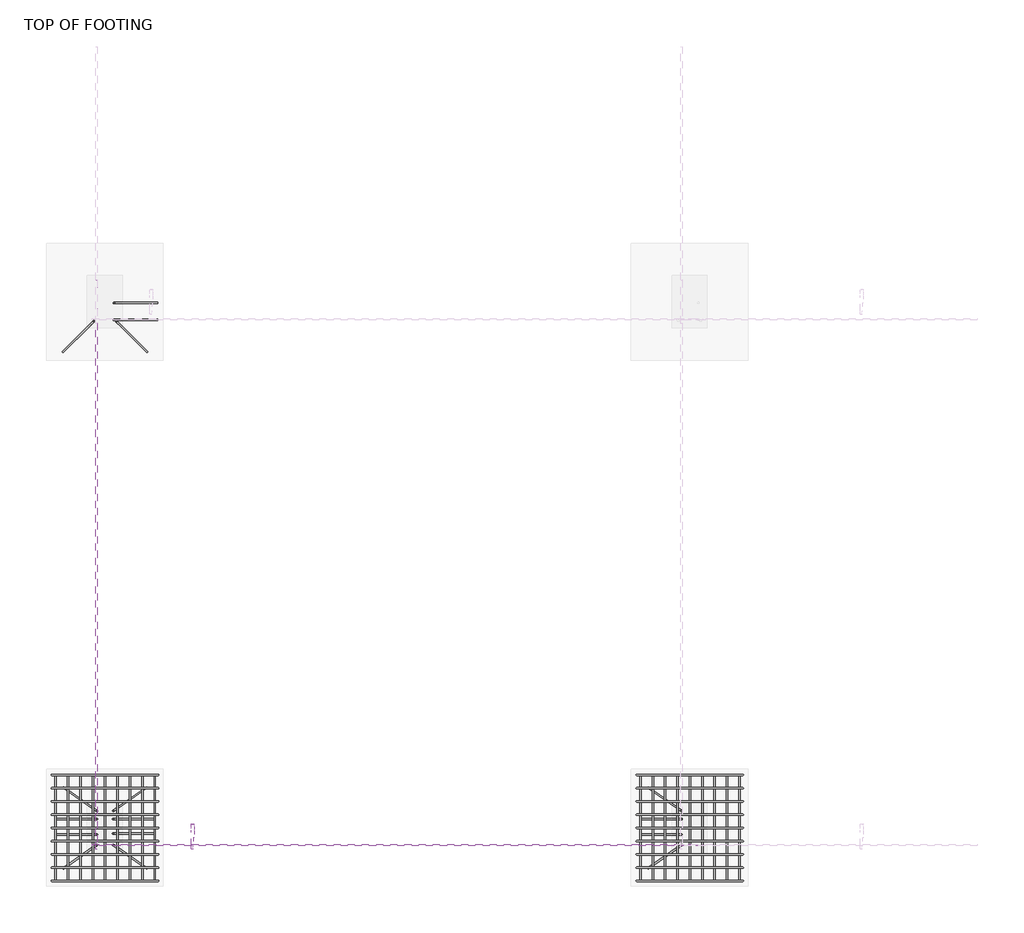
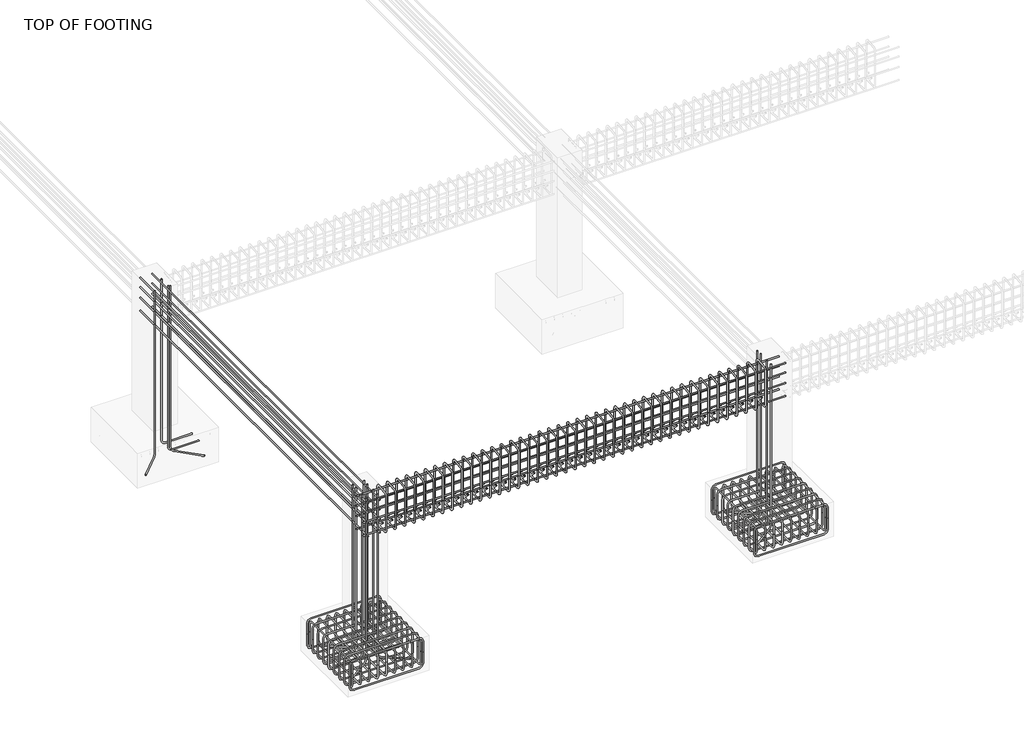
# One storey, part 2 of 13: 29 reinforcing bars.
"""IFC4 building model written with IfcOpenShell, lengths in millimetres."""

from ifc_helpers import new_model, si_unit, point, frame, origin, place, context, project, spatial, polyline, circle_curve, trimmed, segment, composite_curve, source, transform, mapped, element, save
from ifc_brep_helpers import swept_disk

model = new_model("IFC4")

# Units and contexts
model_context = context("Model", 3, world=origin())
ifc_project = project(units=[si_unit("LENGTHUNIT", "METRE", prefix="MILLI")], contexts=[model_context])

# Site, building, storey
site = spatial("IfcSite", under=ifc_project)
building = spatial("IfcBuilding", under=site)
storey = spatial("IfcBuildingStorey", under=building, Name="TOP OF FOOTING", Elevation=-1828.8)

# Reinforcing bars
placement = place(None, origin())
reinforcing_bar_shape = source(origin(), model_context, "Body", "SolidModel", [
    swept_disk(composite_curve([segment(polyline([(-12666.6498378, 3986.1851908, -2049.322685), (-12666.6498378, 3986.1851908, -2196.622685)]), True, "CONTINUOUS"), segment(trimmed(circle_curve(frame((-12712.9998378, 3986.1851908, -2196.622685), z_axis=(0.0, 1.0, 0.0), x_axis=(46.350000000000364, 0.0, 0.0)), 46.35), [point((-12666.6498378, 3986.1851908, -2196.622685))], [point((-12712.9998378, 3986.1851908, -2242.972685))], True, "CARTESIAN"), True, "CONTINUOUS"), segment(polyline([(-12712.9998378, 3986.1851908, -2242.972685), (-13527.5998378, 3986.1851908, -2242.972685)]), True, "CONTINUOUS"), segment(trimmed(circle_curve(frame((-13527.5998378, 3986.1851908, -2196.622685), z_axis=(0.0, 1.0, 0.0), x_axis=(0.0, 0.0, -46.350000000000364)), 46.35), [point((-13527.5998378, 3986.1851908, -2242.972685))], [point((-13573.9498378, 3986.1851908, -2196.622685))], True, "CARTESIAN"), True, "CONTINUOUS"), segment(polyline([(-13573.9498378, 3986.1851908, -2196.622685), (-13573.9498378, 3986.1851908, -2049.322685)]), True, "CONTINUOUS")], self_intersect=False), 6.35),
])
element("IfcReinforcingBar", 1, at=placement, inside=storey, context=model_context, shape_type="MappedRepresentation", body=[
    mapped(reinforcing_bar_shape, transform((0.0, 0.0, 0.0), x_axis=(1.0, 0.0, 0.0), y_axis=(0.0, 1.0, 0.0), z_axis=(0.0, 0.0, 1.0))),
    mapped(reinforcing_bar_shape, transform((0.0, -113.4125, 0.0), x_axis=(1.0, 0.0, 0.0), y_axis=(0.0, 1.0, 0.0), z_axis=(0.0, 0.0, 1.0))),
    mapped(reinforcing_bar_shape, transform((0.0, -226.825, 0.0), x_axis=(1.0, 0.0, 0.0), y_axis=(0.0, 1.0, 0.0), z_axis=(0.0, 0.0, 1.0))),
    mapped(reinforcing_bar_shape, transform((0.0, -340.2375, 0.0), x_axis=(1.0, 0.0, 0.0), y_axis=(0.0, 1.0, 0.0), z_axis=(0.0, 0.0, 1.0))),
    mapped(reinforcing_bar_shape, transform((0.0, -453.65, 0.0), x_axis=(1.0, 0.0, 0.0), y_axis=(0.0, 1.0, 0.0), z_axis=(0.0, 0.0, 1.0))),
    mapped(reinforcing_bar_shape, transform((0.0, -567.0625, 0.0), x_axis=(1.0, 0.0, 0.0), y_axis=(0.0, 1.0, 0.0), z_axis=(0.0, 0.0, 1.0))),
    mapped(reinforcing_bar_shape, transform((0.0, -680.475, 0.0), x_axis=(1.0, 0.0, 0.0), y_axis=(0.0, 1.0, 0.0), z_axis=(0.0, 0.0, 1.0))),
    mapped(reinforcing_bar_shape, transform((0.0, -793.8875, 0.0), x_axis=(1.0, 0.0, 0.0), y_axis=(0.0, 1.0, 0.0), z_axis=(0.0, 0.0, 1.0))),
    mapped(reinforcing_bar_shape, transform((0.0, -907.3, 0.0), x_axis=(1.0, 0.0, 0.0), y_axis=(0.0, 1.0, 0.0), z_axis=(0.0, 0.0, 1.0))),
])
reinforcing_bar_2_shape = source(origin(), model_context, "Body", "SolidModel", [
    swept_disk(composite_curve([segment(polyline([(-13573.9498378, 3986.1851908, -2051.3998363), (-13573.9498378, 3986.1851908, -1904.0998363)]), True, "CONTINUOUS"), segment(trimmed(circle_curve(frame((-13527.5998378, 3986.1851908, -1904.0998363), z_axis=(0.0, 1.0, 0.0), x_axis=(-46.350000000000364, 0.0, 0.0)), 46.35), [point((-13573.9498378, 3986.1851908, -1904.0998363))], [point((-13527.5998378, 3986.1851908, -1857.7498363))], True, "CARTESIAN"), True, "CONTINUOUS"), segment(polyline([(-13527.5998378, 3986.1851908, -1857.7498363), (-12712.9998378, 3986.1851908, -1857.7498363)]), True, "CONTINUOUS"), segment(trimmed(circle_curve(frame((-12712.9998378, 3986.1851908, -1904.0998363), z_axis=(0.0, 1.0, 0.0), x_axis=(0.0, 0.0, 46.350000000000136)), 46.35), [point((-12712.9998378, 3986.1851908, -1857.7498363))], [point((-12666.6498378, 3986.1851908, -1904.0998363))], True, "CARTESIAN"), True, "CONTINUOUS"), segment(polyline([(-12666.6498378, 3986.1851908, -1904.0998363), (-12666.6498378, 3986.1851908, -2051.3998363)]), True, "CONTINUOUS")], self_intersect=False), 6.35),
])
element("IfcReinforcingBar", 2, at=placement, inside=storey, context=model_context, shape_type="MappedRepresentation", body=[
    mapped(reinforcing_bar_2_shape, transform((0.0, 0.0, 0.0), x_axis=(1.0, 0.0, 0.0), y_axis=(0.0, 1.0, 0.0), z_axis=(0.0, 0.0, 1.0))),
    mapped(reinforcing_bar_2_shape, transform((0.0, -113.4125, 0.0), x_axis=(1.0, 0.0, 0.0), y_axis=(0.0, 1.0, 0.0), z_axis=(0.0, 0.0, 1.0))),
    mapped(reinforcing_bar_2_shape, transform((0.0, -226.825, 0.0), x_axis=(1.0, 0.0, 0.0), y_axis=(0.0, 1.0, 0.0), z_axis=(0.0, 0.0, 1.0))),
    mapped(reinforcing_bar_2_shape, transform((0.0, -340.2375, 0.0), x_axis=(1.0, 0.0, 0.0), y_axis=(0.0, 1.0, 0.0), z_axis=(0.0, 0.0, 1.0))),
    mapped(reinforcing_bar_2_shape, transform((0.0, -453.65, 0.0), x_axis=(1.0, 0.0, 0.0), y_axis=(0.0, 1.0, 0.0), z_axis=(0.0, 0.0, 1.0))),
    mapped(reinforcing_bar_2_shape, transform((0.0, -567.0625, 0.0), x_axis=(1.0, 0.0, 0.0), y_axis=(0.0, 1.0, 0.0), z_axis=(0.0, 0.0, 1.0))),
    mapped(reinforcing_bar_2_shape, transform((0.0, -680.475, 0.0), x_axis=(1.0, 0.0, 0.0), y_axis=(0.0, 1.0, 0.0), z_axis=(0.0, 0.0, 1.0))),
    mapped(reinforcing_bar_2_shape, transform((0.0, -793.8875, 0.0), x_axis=(1.0, 0.0, 0.0), y_axis=(0.0, 1.0, 0.0), z_axis=(0.0, 0.0, 1.0))),
    mapped(reinforcing_bar_2_shape, transform((0.0, -907.3, 0.0), x_axis=(1.0, 0.0, 0.0), y_axis=(0.0, 1.0, 0.0), z_axis=(0.0, 0.0, 1.0))),
])
reinforcing_bar_3_shape = source(origin(), model_context, "Body", "SolidModel", [
    swept_disk(composite_curve([segment(polyline([(-13542.4641345, 3986.1851908, -2025.081839), (-13542.4641345, 3986.1851908, -2172.381839)]), True, "CONTINUOUS"), segment(trimmed(circle_curve(frame((-13542.4641345, 3939.8351908, -2172.381839), z_axis=(-1.0, 0.0, 0.0), x_axis=(0.0, 46.34999999999991, 0.0)), 46.35), [point((-13542.4641345, 3986.1851908, -2172.381839))], [point((-13542.4641345, 3939.8351908, -2218.731839))], True, "CARTESIAN"), True, "CONTINUOUS"), segment(polyline([(-13542.4641345, 3939.8351908, -2218.731839), (-13542.4641345, 3125.2351908, -2218.731839)]), True, "CONTINUOUS"), segment(trimmed(circle_curve(frame((-13542.4641345, 3125.2351908, -2172.381839), z_axis=(-1.0, 0.0, 0.0), x_axis=(0.0, 0.0, -46.34999999999991)), 46.35), [point((-13542.4641345, 3125.2351908, -2218.731839))], [point((-13542.4641345, 3078.8851908, -2172.381839))], True, "CARTESIAN"), True, "CONTINUOUS"), segment(polyline([(-13542.4641345, 3078.8851908, -2172.381839), (-13542.4641345, 3078.8851908, -2025.081839)]), True, "CONTINUOUS")], self_intersect=False), 6.35),
])
element("IfcReinforcingBar", 3, at=placement, inside=storey, context=model_context, shape_type="MappedRepresentation", body=[
    mapped(reinforcing_bar_3_shape, transform((0.0, 0.0, 0.0), x_axis=(1.0, 0.0, 0.0), y_axis=(0.0, 1.0, 0.0), z_axis=(0.0, 0.0, 1.0))),
    mapped(reinforcing_bar_3_shape, transform((105.924033, 0.0, 0.0), x_axis=(1.0, 0.0, 0.0), y_axis=(0.0, 1.0, 0.0), z_axis=(0.0, 0.0, 1.0))),
    mapped(reinforcing_bar_3_shape, transform((211.8480661, 0.0, 0.0), x_axis=(1.0, 0.0, 0.0), y_axis=(0.0, 1.0, 0.0), z_axis=(0.0, 0.0, 1.0))),
    mapped(reinforcing_bar_3_shape, transform((317.7720991, 0.0, 0.0), x_axis=(1.0, 0.0, 0.0), y_axis=(0.0, 1.0, 0.0), z_axis=(0.0, 0.0, 1.0))),
    mapped(reinforcing_bar_3_shape, transform((423.6961321, 0.0, 0.0), x_axis=(1.0, 0.0, 0.0), y_axis=(0.0, 1.0, 0.0), z_axis=(0.0, 0.0, 1.0))),
    mapped(reinforcing_bar_3_shape, transform((529.6201652, 0.0, 0.0), x_axis=(1.0, 0.0, 0.0), y_axis=(0.0, 1.0, 0.0), z_axis=(0.0, 0.0, 1.0))),
    mapped(reinforcing_bar_3_shape, transform((635.5441982, 0.0, 0.0), x_axis=(1.0, 0.0, 0.0), y_axis=(0.0, 1.0, 0.0), z_axis=(0.0, 0.0, 1.0))),
    mapped(reinforcing_bar_3_shape, transform((741.4682312, 0.0, 0.0), x_axis=(1.0, 0.0, 0.0), y_axis=(0.0, 1.0, 0.0), z_axis=(0.0, 0.0, 1.0))),
    mapped(reinforcing_bar_3_shape, transform((847.3922643, 0.0, 0.0), x_axis=(1.0, 0.0, 0.0), y_axis=(0.0, 1.0, 0.0), z_axis=(0.0, 0.0, 1.0))),
])
reinforcing_bar_4_shape = source(origin(), model_context, "Body", "SolidModel", [
    swept_disk(composite_curve([segment(polyline([(-12695.0718702, 3986.1851908, -2069.0990329), (-12695.0718702, 3986.1851908, -1921.7990329)]), True, "CONTINUOUS"), segment(trimmed(circle_curve(frame((-12695.0718702, 3939.8351908, -1921.7990329), z_axis=(1.0, 0.0, 0.0), x_axis=(0.0, 46.34999999999991, 0.0)), 46.35), [point((-12695.0718702, 3986.1851908, -1921.7990329))], [point((-12695.0718702, 3939.8351908, -1875.4490329))], True, "CARTESIAN"), True, "CONTINUOUS"), segment(polyline([(-12695.0718702, 3939.8351908, -1875.4490329), (-12695.0718702, 3125.2351908, -1875.4490329)]), True, "CONTINUOUS"), segment(trimmed(circle_curve(frame((-12695.0718702, 3125.2351908, -1921.7990329), z_axis=(1.0, 0.0, 0.0), x_axis=(0.0, 0.0, 46.34999999999991)), 46.35), [point((-12695.0718702, 3125.2351908, -1875.4490329))], [point((-12695.0718702, 3078.8851908, -1921.7990329))], True, "CARTESIAN"), True, "CONTINUOUS"), segment(polyline([(-12695.0718702, 3078.8851908, -1921.7990329), (-12695.0718702, 3078.8851908, -2069.0990329)]), True, "CONTINUOUS")], self_intersect=False), 6.35),
])
element("IfcReinforcingBar", 4, at=placement, inside=storey, context=model_context, shape_type="MappedRepresentation", body=[
    mapped(reinforcing_bar_4_shape, transform((0.0, 0.0, 0.0), x_axis=(1.0, 0.0, 0.0), y_axis=(0.0, 1.0, 0.0), z_axis=(0.0, 0.0, 1.0))),
    mapped(reinforcing_bar_4_shape, transform((-105.924033, 0.0, 0.0), x_axis=(1.0, 0.0, 0.0), y_axis=(0.0, 1.0, 0.0), z_axis=(0.0, 0.0, 1.0))),
    mapped(reinforcing_bar_4_shape, transform((-211.8480661, 0.0, 0.0), x_axis=(1.0, 0.0, 0.0), y_axis=(0.0, 1.0, 0.0), z_axis=(0.0, 0.0, 1.0))),
    mapped(reinforcing_bar_4_shape, transform((-317.7720991, 0.0, 0.0), x_axis=(1.0, 0.0, 0.0), y_axis=(0.0, 1.0, 0.0), z_axis=(0.0, 0.0, 1.0))),
    mapped(reinforcing_bar_4_shape, transform((-423.6961321, 0.0, 0.0), x_axis=(1.0, 0.0, 0.0), y_axis=(0.0, 1.0, 0.0), z_axis=(0.0, 0.0, 1.0))),
    mapped(reinforcing_bar_4_shape, transform((-529.6201652, 0.0, 0.0), x_axis=(1.0, 0.0, 0.0), y_axis=(0.0, 1.0, 0.0), z_axis=(0.0, 0.0, 1.0))),
    mapped(reinforcing_bar_4_shape, transform((-635.5441982, 0.0, 0.0), x_axis=(1.0, 0.0, 0.0), y_axis=(0.0, 1.0, 0.0), z_axis=(0.0, 0.0, 1.0))),
    mapped(reinforcing_bar_4_shape, transform((-741.4682312, 0.0, 0.0), x_axis=(1.0, 0.0, 0.0), y_axis=(0.0, 1.0, 0.0), z_axis=(0.0, 0.0, 1.0))),
    mapped(reinforcing_bar_4_shape, transform((-847.3922643, 0.0, 0.0), x_axis=(1.0, 0.0, 0.0), y_axis=(0.0, 1.0, 0.0), z_axis=(0.0, 0.0, 1.0))),
])
reinforcing_bar_5_shape = source(origin(), model_context, "Body", "SolidModel", [
    swept_disk(composite_curve([segment(polyline([(-7666.6498378, 3986.1851908, -2049.322685), (-7666.6498378, 3986.1851908, -2196.622685)]), True, "CONTINUOUS"), segment(trimmed(circle_curve(frame((-7712.9998378, 3986.1851908, -2196.622685), z_axis=(0.0, 1.0, 0.0), x_axis=(46.350000000000364, 0.0, 0.0)), 46.35), [point((-7666.6498378, 3986.1851908, -2196.622685))], [point((-7712.9998378, 3986.1851908, -2242.972685))], True, "CARTESIAN"), True, "CONTINUOUS"), segment(polyline([(-7712.9998378, 3986.1851908, -2242.972685), (-8527.5998378, 3986.1851908, -2242.972685)]), True, "CONTINUOUS"), segment(trimmed(circle_curve(frame((-8527.5998378, 3986.1851908, -2196.622685), z_axis=(0.0, 1.0, 0.0), x_axis=(0.0, 0.0, -46.350000000000364)), 46.35), [point((-8527.5998378, 3986.1851908, -2242.972685))], [point((-8573.9498378, 3986.1851908, -2196.622685))], True, "CARTESIAN"), True, "CONTINUOUS"), segment(polyline([(-8573.9498378, 3986.1851908, -2196.622685), (-8573.9498378, 3986.1851908, -2049.322685)]), True, "CONTINUOUS")], self_intersect=False), 6.35),
])
element("IfcReinforcingBar", 5, at=placement, inside=storey, context=model_context, shape_type="MappedRepresentation", body=[
    mapped(reinforcing_bar_5_shape, transform((0.0, 0.0, 0.0), x_axis=(1.0, 0.0, 0.0), y_axis=(0.0, 1.0, 0.0), z_axis=(0.0, 0.0, 1.0))),
    mapped(reinforcing_bar_5_shape, transform((0.0, -113.4125, 0.0), x_axis=(1.0, 0.0, 0.0), y_axis=(0.0, 1.0, 0.0), z_axis=(0.0, 0.0, 1.0))),
    mapped(reinforcing_bar_5_shape, transform((0.0, -226.825, 0.0), x_axis=(1.0, 0.0, 0.0), y_axis=(0.0, 1.0, 0.0), z_axis=(0.0, 0.0, 1.0))),
    mapped(reinforcing_bar_5_shape, transform((0.0, -340.2375, 0.0), x_axis=(1.0, 0.0, 0.0), y_axis=(0.0, 1.0, 0.0), z_axis=(0.0, 0.0, 1.0))),
    mapped(reinforcing_bar_5_shape, transform((0.0, -453.65, 0.0), x_axis=(1.0, 0.0, 0.0), y_axis=(0.0, 1.0, 0.0), z_axis=(0.0, 0.0, 1.0))),
    mapped(reinforcing_bar_5_shape, transform((0.0, -567.0625, 0.0), x_axis=(1.0, 0.0, 0.0), y_axis=(0.0, 1.0, 0.0), z_axis=(0.0, 0.0, 1.0))),
    mapped(reinforcing_bar_5_shape, transform((0.0, -680.475, 0.0), x_axis=(1.0, 0.0, 0.0), y_axis=(0.0, 1.0, 0.0), z_axis=(0.0, 0.0, 1.0))),
    mapped(reinforcing_bar_5_shape, transform((0.0, -793.8875, 0.0), x_axis=(1.0, 0.0, 0.0), y_axis=(0.0, 1.0, 0.0), z_axis=(0.0, 0.0, 1.0))),
    mapped(reinforcing_bar_5_shape, transform((0.0, -907.3, 0.0), x_axis=(1.0, 0.0, 0.0), y_axis=(0.0, 1.0, 0.0), z_axis=(0.0, 0.0, 1.0))),
])
reinforcing_bar_6_shape = source(origin(), model_context, "Body", "SolidModel", [
    swept_disk(composite_curve([segment(polyline([(-8573.9498378, 3986.1851908, -2051.3998363), (-8573.9498378, 3986.1851908, -1904.0998363)]), True, "CONTINUOUS"), segment(trimmed(circle_curve(frame((-8527.5998378, 3986.1851908, -1904.0998363), z_axis=(0.0, 1.0, 0.0), x_axis=(-46.350000000000364, 0.0, 0.0)), 46.35), [point((-8573.9498378, 3986.1851908, -1904.0998363))], [point((-8527.5998378, 3986.1851908, -1857.7498363))], True, "CARTESIAN"), True, "CONTINUOUS"), segment(polyline([(-8527.5998378, 3986.1851908, -1857.7498363), (-7712.9998378, 3986.1851908, -1857.7498363)]), True, "CONTINUOUS"), segment(trimmed(circle_curve(frame((-7712.9998378, 3986.1851908, -1904.0998363), z_axis=(0.0, 1.0, 0.0), x_axis=(0.0, 0.0, 46.350000000000136)), 46.35), [point((-7712.9998378, 3986.1851908, -1857.7498363))], [point((-7666.6498378, 3986.1851908, -1904.0998363))], True, "CARTESIAN"), True, "CONTINUOUS"), segment(polyline([(-7666.6498378, 3986.1851908, -1904.0998363), (-7666.6498378, 3986.1851908, -2051.3998363)]), True, "CONTINUOUS")], self_intersect=False), 6.35),
])
element("IfcReinforcingBar", 6, at=placement, inside=storey, context=model_context, shape_type="MappedRepresentation", body=[
    mapped(reinforcing_bar_6_shape, transform((0.0, 0.0, 0.0), x_axis=(1.0, 0.0, 0.0), y_axis=(0.0, 1.0, 0.0), z_axis=(0.0, 0.0, 1.0))),
    mapped(reinforcing_bar_6_shape, transform((0.0, -113.4125, 0.0), x_axis=(1.0, 0.0, 0.0), y_axis=(0.0, 1.0, 0.0), z_axis=(0.0, 0.0, 1.0))),
    mapped(reinforcing_bar_6_shape, transform((0.0, -226.825, 0.0), x_axis=(1.0, 0.0, 0.0), y_axis=(0.0, 1.0, 0.0), z_axis=(0.0, 0.0, 1.0))),
    mapped(reinforcing_bar_6_shape, transform((0.0, -340.2375, 0.0), x_axis=(1.0, 0.0, 0.0), y_axis=(0.0, 1.0, 0.0), z_axis=(0.0, 0.0, 1.0))),
    mapped(reinforcing_bar_6_shape, transform((0.0, -453.65, 0.0), x_axis=(1.0, 0.0, 0.0), y_axis=(0.0, 1.0, 0.0), z_axis=(0.0, 0.0, 1.0))),
    mapped(reinforcing_bar_6_shape, transform((0.0, -567.0625, 0.0), x_axis=(1.0, 0.0, 0.0), y_axis=(0.0, 1.0, 0.0), z_axis=(0.0, 0.0, 1.0))),
    mapped(reinforcing_bar_6_shape, transform((0.0, -680.475, 0.0), x_axis=(1.0, 0.0, 0.0), y_axis=(0.0, 1.0, 0.0), z_axis=(0.0, 0.0, 1.0))),
    mapped(reinforcing_bar_6_shape, transform((0.0, -793.8875, 0.0), x_axis=(1.0, 0.0, 0.0), y_axis=(0.0, 1.0, 0.0), z_axis=(0.0, 0.0, 1.0))),
    mapped(reinforcing_bar_6_shape, transform((0.0, -907.3, 0.0), x_axis=(1.0, 0.0, 0.0), y_axis=(0.0, 1.0, 0.0), z_axis=(0.0, 0.0, 1.0))),
])
reinforcing_bar_7_shape = source(origin(), model_context, "Body", "SolidModel", [
    swept_disk(composite_curve([segment(polyline([(-8542.4641345, 3986.1851908, -2025.081839), (-8542.4641345, 3986.1851908, -2172.381839)]), True, "CONTINUOUS"), segment(trimmed(circle_curve(frame((-8542.4641345, 3939.8351908, -2172.381839), z_axis=(-1.0, 0.0, 0.0), x_axis=(0.0, 46.34999999999991, 0.0)), 46.35), [point((-8542.4641345, 3986.1851908, -2172.381839))], [point((-8542.4641345, 3939.8351908, -2218.731839))], True, "CARTESIAN"), True, "CONTINUOUS"), segment(polyline([(-8542.4641345, 3939.8351908, -2218.731839), (-8542.4641345, 3125.2351908, -2218.731839)]), True, "CONTINUOUS"), segment(trimmed(circle_curve(frame((-8542.4641345, 3125.2351908, -2172.381839), z_axis=(-1.0, 0.0, 0.0), x_axis=(0.0, 0.0, -46.34999999999991)), 46.35), [point((-8542.4641345, 3125.2351908, -2218.731839))], [point((-8542.4641345, 3078.8851908, -2172.381839))], True, "CARTESIAN"), True, "CONTINUOUS"), segment(polyline([(-8542.4641345, 3078.8851908, -2172.381839), (-8542.4641345, 3078.8851908, -2025.081839)]), True, "CONTINUOUS")], self_intersect=False), 6.35),
])
element("IfcReinforcingBar", 7, at=placement, inside=storey, context=model_context, shape_type="MappedRepresentation", body=[
    mapped(reinforcing_bar_7_shape, transform((0.0, 0.0, 0.0), x_axis=(1.0, 0.0, 0.0), y_axis=(0.0, 1.0, 0.0), z_axis=(0.0, 0.0, 1.0))),
    mapped(reinforcing_bar_7_shape, transform((105.924033, 0.0, 0.0), x_axis=(1.0, 0.0, 0.0), y_axis=(0.0, 1.0, 0.0), z_axis=(0.0, 0.0, 1.0))),
    mapped(reinforcing_bar_7_shape, transform((211.8480661, 0.0, 0.0), x_axis=(1.0, 0.0, 0.0), y_axis=(0.0, 1.0, 0.0), z_axis=(0.0, 0.0, 1.0))),
    mapped(reinforcing_bar_7_shape, transform((317.7720991, 0.0, 0.0), x_axis=(1.0, 0.0, 0.0), y_axis=(0.0, 1.0, 0.0), z_axis=(0.0, 0.0, 1.0))),
    mapped(reinforcing_bar_7_shape, transform((423.6961321, 0.0, 0.0), x_axis=(1.0, 0.0, 0.0), y_axis=(0.0, 1.0, 0.0), z_axis=(0.0, 0.0, 1.0))),
    mapped(reinforcing_bar_7_shape, transform((529.6201652, 0.0, 0.0), x_axis=(1.0, 0.0, 0.0), y_axis=(0.0, 1.0, 0.0), z_axis=(0.0, 0.0, 1.0))),
    mapped(reinforcing_bar_7_shape, transform((635.5441982, 0.0, 0.0), x_axis=(1.0, 0.0, 0.0), y_axis=(0.0, 1.0, 0.0), z_axis=(0.0, 0.0, 1.0))),
    mapped(reinforcing_bar_7_shape, transform((741.4682312, 0.0, 0.0), x_axis=(1.0, 0.0, 0.0), y_axis=(0.0, 1.0, 0.0), z_axis=(0.0, 0.0, 1.0))),
    mapped(reinforcing_bar_7_shape, transform((847.3922643, 0.0, 0.0), x_axis=(1.0, 0.0, 0.0), y_axis=(0.0, 1.0, 0.0), z_axis=(0.0, 0.0, 1.0))),
])
reinforcing_bar_8_shape = source(origin(), model_context, "Body", "SolidModel", [
    swept_disk(composite_curve([segment(polyline([(-7695.0718702, 3986.1851908, -2069.0990329), (-7695.0718702, 3986.1851908, -1921.7990329)]), True, "CONTINUOUS"), segment(trimmed(circle_curve(frame((-7695.0718702, 3939.8351908, -1921.7990329), z_axis=(1.0, 0.0, 0.0), x_axis=(0.0, 46.34999999999991, 0.0)), 46.35), [point((-7695.0718702, 3986.1851908, -1921.7990329))], [point((-7695.0718702, 3939.8351908, -1875.4490329))], True, "CARTESIAN"), True, "CONTINUOUS"), segment(polyline([(-7695.0718702, 3939.8351908, -1875.4490329), (-7695.0718702, 3125.2351908, -1875.4490329)]), True, "CONTINUOUS"), segment(trimmed(circle_curve(frame((-7695.0718702, 3125.2351908, -1921.7990329), z_axis=(1.0, 0.0, 0.0), x_axis=(0.0, 0.0, 46.34999999999991)), 46.35), [point((-7695.0718702, 3125.2351908, -1875.4490329))], [point((-7695.0718702, 3078.8851908, -1921.7990329))], True, "CARTESIAN"), True, "CONTINUOUS"), segment(polyline([(-7695.0718702, 3078.8851908, -1921.7990329), (-7695.0718702, 3078.8851908, -2069.0990329)]), True, "CONTINUOUS")], self_intersect=False), 6.35),
])
element("IfcReinforcingBar", 8, at=placement, inside=storey, context=model_context, shape_type="MappedRepresentation", body=[
    mapped(reinforcing_bar_8_shape, transform((0.0, 0.0, 0.0), x_axis=(1.0, 0.0, 0.0), y_axis=(0.0, 1.0, 0.0), z_axis=(0.0, 0.0, 1.0))),
    mapped(reinforcing_bar_8_shape, transform((-105.924033, 0.0, 0.0), x_axis=(1.0, 0.0, 0.0), y_axis=(0.0, 1.0, 0.0), z_axis=(0.0, 0.0, 1.0))),
    mapped(reinforcing_bar_8_shape, transform((-211.8480661, 0.0, 0.0), x_axis=(1.0, 0.0, 0.0), y_axis=(0.0, 1.0, 0.0), z_axis=(0.0, 0.0, 1.0))),
    mapped(reinforcing_bar_8_shape, transform((-317.7720991, 0.0, 0.0), x_axis=(1.0, 0.0, 0.0), y_axis=(0.0, 1.0, 0.0), z_axis=(0.0, 0.0, 1.0))),
    mapped(reinforcing_bar_8_shape, transform((-423.6961321, 0.0, 0.0), x_axis=(1.0, 0.0, 0.0), y_axis=(0.0, 1.0, 0.0), z_axis=(0.0, 0.0, 1.0))),
    mapped(reinforcing_bar_8_shape, transform((-529.6201652, 0.0, 0.0), x_axis=(1.0, 0.0, 0.0), y_axis=(0.0, 1.0, 0.0), z_axis=(0.0, 0.0, 1.0))),
    mapped(reinforcing_bar_8_shape, transform((-635.5441982, 0.0, 0.0), x_axis=(1.0, 0.0, 0.0), y_axis=(0.0, 1.0, 0.0), z_axis=(0.0, 0.0, 1.0))),
    mapped(reinforcing_bar_8_shape, transform((-741.4682312, 0.0, 0.0), x_axis=(1.0, 0.0, 0.0), y_axis=(0.0, 1.0, 0.0), z_axis=(0.0, 0.0, 1.0))),
    mapped(reinforcing_bar_8_shape, transform((-847.3922643, 0.0, 0.0), x_axis=(1.0, 0.0, 0.0), y_axis=(0.0, 1.0, 0.0), z_axis=(0.0, 0.0, 1.0))),
])
reinforcing_bar_9_shape = source(origin(), model_context, "Body", "SolidModel", [
    swept_disk(composite_curve([segment(polyline([(-13044.6810723, 8023.2621018, -40.0), (-13044.6810723, 8023.2621018, -2147.4714407)]), True, "CONTINUOUS"), segment(trimmed(circle_curve(frame((-12998.3310723, 8023.2621018, -2147.4714407), z_axis=(0.0, -1.0, 0.0), x_axis=(-46.350000000000364, 0.0, 0.0)), 46.35), [point((-13044.6810723, 8023.2621018, -2147.4714407))], [point((-12998.3310723, 8023.2621018, -2193.8214407))], True, "CARTESIAN"), True, "CONTINUOUS"), segment(polyline([(-12998.3310723, 8023.2621018, -2193.8214407), (-12667.4997506, 8023.2621018, -2193.8214407)]), True, "CONTINUOUS")], self_intersect=False), 6.35),
])
element("IfcReinforcingBar", 9, at=placement, inside=storey, context=model_context, shape_type="MappedRepresentation", body=[
    mapped(reinforcing_bar_9_shape, transform((0.0, 0.0, 0.0), x_axis=(1.0, 0.0, 0.0), y_axis=(0.0, 1.0, 0.0), z_axis=(0.0, 0.0, 1.0))),
    mapped(reinforcing_bar_9_shape, transform((0.0, -144.620853, 0.0), x_axis=(1.0, 0.0, 0.0), y_axis=(0.0, 1.0, 0.0), z_axis=(0.0, 0.0, 1.0))),
])
element("IfcReinforcingBar", 10, at=placement, inside=storey, context=model_context, shape_type="SolidModel", body=[
    swept_disk(composite_curve([segment(polyline([(-13024.6810723, 7868.8851908, -40.0), (-13024.6810723, 7868.8851908, -2147.4714407)]), True, "CONTINUOUS"), segment(trimmed(circle_curve(frame((-12991.906673, 7836.1107915, -2147.4714407), z_axis=(-0.7071067811865542, -0.7071067811865408, 0.0), x_axis=(-32.77439930000037, 32.77439929999946, 0.0)), 46.35), [point((-13024.6810723, 7868.8851908, -2147.4714407))], [point((-12991.906673, 7836.1107915, -2193.8214407))], True, "CARTESIAN"), True, "CONTINUOUS"), segment(polyline([(-12991.906673, 7836.1107915, -2193.8214407), (-12757.973602, 7602.1777205, -2193.8214407)]), True, "CONTINUOUS")], self_intersect=False), 6.35),
])
element("IfcReinforcingBar", 11, at=placement, inside=storey, context=model_context, shape_type="SolidModel", body=[
    swept_disk(composite_curve([segment(polyline([(-13215.9186034, 7868.8851908, -40.0), (-13215.9186034, 7868.8851908, -2147.4714407)]), True, "CONTINUOUS"), segment(trimmed(circle_curve(frame((-13248.6930027, 7836.1107915, -2147.4714407), z_axis=(-0.7071067811865339, 0.7071067811865611, 0.0), x_axis=(32.77439930000037, 32.77439929999946, 0.0)), 46.35), [point((-13215.9186034, 7868.8851908, -2147.4714407))], [point((-13248.6930027, 7836.1107915, -2193.8214407))], True, "CARTESIAN"), True, "CONTINUOUS"), segment(polyline([(-13248.6930027, 7836.1107915, -2193.8214407), (-13482.6260737, 7602.1777205, -2193.8214407)]), True, "CONTINUOUS")], self_intersect=False), 6.35),
])
reinforcing_bar_10_shape = source(origin(), model_context, "Body", "SolidModel", [
    swept_disk(composite_curve([segment(polyline([(-8190.3202778, 3474.1031528, -40.0), (-8190.3202778, 3474.1031528, -2122.45)]), True, "CONTINUOUS"), segment(trimmed(circle_curve(frame((-8236.6702778, 3474.1031528, -2122.45), z_axis=(0.0, 1.0, 0.0), x_axis=(46.349999999999454, 0.0, 0.0)), 46.35), [point((-8190.3202778, 3474.1031528, -2122.45))], [point((-8236.6702778, 3474.1031528, -2168.8))], True, "CARTESIAN"), True, "CONTINUOUS"), segment(polyline([(-8236.6702778, 3474.1031528, -2168.8), (-8542.4641345, 3474.1031528, -2168.8)]), True, "CONTINUOUS")], self_intersect=False), 6.35),
])
element("IfcReinforcingBar", 12, at=placement, inside=storey, context=model_context, shape_type="MappedRepresentation", body=[
    mapped(reinforcing_bar_10_shape, transform((0.0, 0.0, 0.0), x_axis=(1.0, 0.0, 0.0), y_axis=(0.0, 1.0, 0.0), z_axis=(0.0, 0.0, 1.0))),
    mapped(reinforcing_bar_10_shape, transform((0.0, 133.432038, 0.0), x_axis=(1.0, 0.0, 0.0), y_axis=(0.0, 1.0, 0.0), z_axis=(0.0, 0.0, 1.0))),
])
element("IfcReinforcingBar", 13, at=placement, inside=storey, context=model_context, shape_type="SolidModel", body=[
    swept_disk(composite_curve([segment(polyline([(-8190.3202778, 3386.5851908, -40.0), (-8190.3202778, 3386.5851908, -2122.45)]), True, "CONTINUOUS"), segment(trimmed(circle_curve(frame((-8228.2879751, 3359.999923, -2122.45), z_axis=(-0.5735764363510439, 0.8191520442889934, 0.0), x_axis=(37.9676972999996, 26.58526780000011, 0.0)), 46.35), [point((-8190.3202778, 3386.5851908, -2122.45))], [point((-8228.2879751, 3359.999923, -2168.8))], True, "CARTESIAN"), True, "CONTINUOUS"), segment(polyline([(-8228.2879751, 3359.999923, -2168.8), (-8478.7796379, 3184.6037724, -2168.8)]), True, "CONTINUOUS")], self_intersect=False), 6.35),
])
element("IfcReinforcingBar", 14, at=placement, inside=storey, context=model_context, shape_type="SolidModel", body=[
    swept_disk(composite_curve([segment(polyline([(-8190.3202778, 3678.4851908, -40.0), (-8190.3202778, 3678.4851908, -2122.45)]), True, "CONTINUOUS"), segment(trimmed(circle_curve(frame((-8228.2879751, 3705.0704586, -2122.45), z_axis=(0.5735764363510498, 0.8191520442889892, 0.0), x_axis=(37.9676972999996, -26.58526780000011, 0.0)), 46.35), [point((-8190.3202778, 3678.4851908, -2122.45))], [point((-8228.2879751, 3705.0704586, -2168.8))], True, "CARTESIAN"), True, "CONTINUOUS"), segment(polyline([(-8228.2879751, 3705.0704586, -2168.8), (-8478.7796379, 3880.4666092, -2168.8)]), True, "CONTINUOUS")], self_intersect=False), 6.35),
])
reinforcing_bar_11_shape = source(origin(), model_context, "Body", "SolidModel", [
    swept_disk(composite_curve([segment(polyline([(-13190.3202778, 3474.1031528, -40.0), (-13190.3202778, 3474.1031528, -2122.45)]), True, "CONTINUOUS"), segment(trimmed(circle_curve(frame((-13236.6702778, 3474.1031528, -2122.45), z_axis=(0.0, 1.0, 0.0), x_axis=(46.350000000000364, 0.0, 0.0)), 46.35), [point((-13190.3202778, 3474.1031528, -2122.45))], [point((-13236.6702778, 3474.1031528, -2168.8))], True, "CARTESIAN"), True, "CONTINUOUS"), segment(polyline([(-13236.6702778, 3474.1031528, -2168.8), (-13542.4641345, 3474.1031528, -2168.8)]), True, "CONTINUOUS")], self_intersect=False), 6.35),
])
element("IfcReinforcingBar", 15, at=placement, inside=storey, context=model_context, shape_type="MappedRepresentation", body=[
    mapped(reinforcing_bar_11_shape, transform((0.0, 0.0, 0.0), x_axis=(1.0, 0.0, 0.0), y_axis=(0.0, 1.0, 0.0), z_axis=(0.0, 0.0, 1.0))),
    mapped(reinforcing_bar_11_shape, transform((0.0, 133.432038, 0.0), x_axis=(1.0, 0.0, 0.0), y_axis=(0.0, 1.0, 0.0), z_axis=(0.0, 0.0, 1.0))),
])
element("IfcReinforcingBar", 16, at=placement, inside=storey, context=model_context, shape_type="SolidModel", body=[
    swept_disk(composite_curve([segment(polyline([(-13190.3202778, 3386.5851908, -40.0), (-13190.3202778, 3386.5851908, -2122.45)]), True, "CONTINUOUS"), segment(trimmed(circle_curve(frame((-13228.2879751, 3359.999923, -2122.45), z_axis=(-0.5735764363510439, 0.8191520442889934, 0.0), x_axis=(37.96769730000051, 26.58526780000011, 0.0)), 46.35), [point((-13190.3202778, 3386.5851908, -2122.45))], [point((-13228.2879751, 3359.999923, -2168.8))], True, "CARTESIAN"), True, "CONTINUOUS"), segment(polyline([(-13228.2879751, 3359.999923, -2168.8), (-13478.7796379, 3184.6037724, -2168.8)]), True, "CONTINUOUS")], self_intersect=False), 6.35),
])
element("IfcReinforcingBar", 17, at=placement, inside=storey, context=model_context, shape_type="SolidModel", body=[
    swept_disk(composite_curve([segment(polyline([(-13050.2793979, 3386.5851908, -40.0), (-13050.2793979, 3386.5851908, -2122.45)]), True, "CONTINUOUS"), segment(trimmed(circle_curve(frame((-13012.3117006, 3359.999923, -2122.45), z_axis=(-0.5735764363510439, -0.8191520442889934, 0.0), x_axis=(-37.96769730000051, 26.58526780000011, 0.0)), 46.35), [point((-13050.2793979, 3386.5851908, -2122.45))], [point((-13012.3117006, 3359.999923, -2168.8))], True, "CARTESIAN"), True, "CONTINUOUS"), segment(polyline([(-13012.3117006, 3359.999923, -2168.8), (-12761.8200378, 3184.6037724, -2168.8)]), True, "CONTINUOUS")], self_intersect=False), 6.35),
])
element("IfcReinforcingBar", 18, at=placement, inside=storey, context=model_context, shape_type="SolidModel", body=[
    swept_disk(composite_curve([segment(polyline([(-13190.3202778, 3678.4851908, -40.0), (-13190.3202778, 3678.4851908, -2122.45)]), True, "CONTINUOUS"), segment(trimmed(circle_curve(frame((-13228.2879751, 3705.0704586, -2122.45), z_axis=(0.5735764363510498, 0.8191520442889892, 0.0), x_axis=(37.96769730000051, -26.58526780000011, 0.0)), 46.35), [point((-13190.3202778, 3678.4851908, -2122.45))], [point((-13228.2879751, 3705.0704586, -2168.8))], True, "CARTESIAN"), True, "CONTINUOUS"), segment(polyline([(-13228.2879751, 3705.0704586, -2168.8), (-13478.7796379, 3880.4666092, -2168.8)]), True, "CONTINUOUS")], self_intersect=False), 6.35),
])
element("IfcReinforcingBar", 19, at=placement, inside=storey, context=model_context, shape_type="SolidModel", body=[
    swept_disk(composite_curve([segment(polyline([(-13050.2793979, 3678.4851908, -40.0), (-13050.2793979, 3678.4851908, -2122.45)]), True, "CONTINUOUS"), segment(trimmed(circle_curve(frame((-13012.3117006, 3705.0704586, -2122.45), z_axis=(0.573576436351038, -0.8191520442889975, 0.0), x_axis=(-37.96769730000051, -26.58526780000011, 0.0)), 46.35), [point((-13050.2793979, 3678.4851908, -2122.45))], [point((-13012.3117006, 3705.0704586, -2168.8))], True, "CARTESIAN"), True, "CONTINUOUS"), segment(polyline([(-13012.3117006, 3705.0704586, -2168.8), (-12761.8200378, 3880.4666092, -2168.8)]), True, "CONTINUOUS")], self_intersect=False), 6.35),
])
reinforcing_bar_12_shape = source(origin(), model_context, "Body", "SolidModel", [
    swept_disk(composite_curve([segment(polyline([(-13050.2793979, 3607.5351908, -40.0), (-13050.2793979, 3607.5351908, -2122.45)]), True, "CONTINUOUS"), segment(trimmed(circle_curve(frame((-13003.9293979, 3607.5351908, -2122.45), z_axis=(0.0, -1.0, 0.0), x_axis=(-46.350000000000364, 0.0, 0.0)), 46.35), [point((-13050.2793979, 3607.5351908, -2122.45))], [point((-13003.9293979, 3607.5351908, -2168.8))], True, "CARTESIAN"), True, "CONTINUOUS"), segment(polyline([(-13003.9293979, 3607.5351908, -2168.8), (-12697.3985869, 3607.5351908, -2168.8)]), True, "CONTINUOUS")], self_intersect=False), 6.35),
])
element("IfcReinforcingBar", 20, at=placement, inside=storey, context=model_context, shape_type="MappedRepresentation", body=[
    mapped(reinforcing_bar_12_shape, transform((0.0, 0.0, 0.0), x_axis=(1.0, 0.0, 0.0), y_axis=(0.0, 1.0, 0.0), z_axis=(0.0, 0.0, 1.0))),
    mapped(reinforcing_bar_12_shape, transform((0.0, -124.205444, 0.0), x_axis=(1.0, 0.0, 0.0), y_axis=(0.0, 1.0, 0.0), z_axis=(0.0, 0.0, 1.0))),
])
reinforcing_bar_13_shape = source(origin(), model_context, "Body", "SolidModel", [
    swept_disk(composite_curve([segment(polyline([(-13192.6754021, 3347.5351908, -87.6047527), (-13192.6754021, 8217.5351908, -87.6047527)]), True, "CONTINUOUS")], self_intersect=False), 6.35),
])
element("IfcReinforcingBar", 21, at=placement, inside=storey, context=model_context, shape_type="MappedRepresentation", body=[
    mapped(reinforcing_bar_13_shape, transform((0.0, 0.0, 0.0), x_axis=(1.0, 0.0, 0.0), y_axis=(0.0, 1.0, 0.0), z_axis=(0.0, 0.0, 1.0))),
    mapped(reinforcing_bar_13_shape, transform((144.710816, 0.0, 0.0), x_axis=(1.0, 0.0, 0.0), y_axis=(0.0, 1.0, 0.0), z_axis=(0.0, 0.0, 1.0))),
])
reinforcing_bar_14_shape = source(origin(), model_context, "Body", "SolidModel", [
    swept_disk(composite_curve([segment(polyline([(-13192.6754021, 3347.5351908, -212.6047527), (-13192.6754021, 8217.5351908, -212.6047527)]), True, "CONTINUOUS")], self_intersect=False), 6.35),
])
element("IfcReinforcingBar", 22, at=placement, inside=storey, context=model_context, shape_type="MappedRepresentation", body=[
    mapped(reinforcing_bar_14_shape, transform((0.0, 0.0, 0.0), x_axis=(1.0, 0.0, 0.0), y_axis=(0.0, 1.0, 0.0), z_axis=(0.0, 0.0, 1.0))),
    mapped(reinforcing_bar_14_shape, transform((144.710816, 0.0, 0.0), x_axis=(1.0, 0.0, 0.0), y_axis=(0.0, 1.0, 0.0), z_axis=(0.0, 0.0, 1.0))),
])
reinforcing_bar_15_shape = source(origin(), model_context, "Body", "SolidModel", [
    swept_disk(composite_curve([segment(polyline([(-13192.6754021, 3347.5351908, -517.6047527), (-13192.6754021, 8217.5351908, -517.6047527)]), True, "CONTINUOUS")], self_intersect=False), 6.35),
])
element("IfcReinforcingBar", 23, at=placement, inside=storey, context=model_context, shape_type="MappedRepresentation", body=[
    mapped(reinforcing_bar_15_shape, transform((0.0, 0.0, 0.0), x_axis=(1.0, 0.0, 0.0), y_axis=(0.0, 1.0, 0.0), z_axis=(0.0, 0.0, 1.0))),
    mapped(reinforcing_bar_15_shape, transform((144.710816, 0.0, 0.0), x_axis=(1.0, 0.0, 0.0), y_axis=(0.0, 1.0, 0.0), z_axis=(0.0, 0.0, 1.0))),
])
reinforcing_bar_16_shape = source(origin(), model_context, "Body", "SolidModel", [
    swept_disk(composite_curve([segment(polyline([(-13192.6754021, 3347.5351908, -347.6047527), (-13192.6754021, 8217.5351908, -347.6047527)]), True, "CONTINUOUS")], self_intersect=False), 6.35),
])
element("IfcReinforcingBar", 24, at=placement, inside=storey, context=model_context, shape_type="MappedRepresentation", body=[
    mapped(reinforcing_bar_16_shape, transform((0.0, 0.0, 0.0), x_axis=(1.0, 0.0, 0.0), y_axis=(0.0, 1.0, 0.0), z_axis=(0.0, 0.0, 1.0))),
    mapped(reinforcing_bar_16_shape, transform((144.710816, 0.0, 0.0), x_axis=(1.0, 0.0, 0.0), y_axis=(0.0, 1.0, 0.0), z_axis=(0.0, 0.0, 1.0))),
])
reinforcing_bar_17_shape = source(origin(), model_context, "Body", "SolidModel", [
    swept_disk(composite_curve([segment(polyline([(-8276.6498378, 3496.2594254, -444.3886395), (-8276.6498378, 3552.0029884, -500.1322024)]), True, "CONTINUOUS"), segment(trimmed(circle_curve(frame((-8276.6498378, 3529.8351908, -522.3), z_axis=(-1.0, 0.0, 0.0), x_axis=(0.0, 22.167797600000085, 22.16779759999997)), 31.35), [point((-8276.6498378, 3552.0029884, -500.1322024))], [point((-8276.6498378, 3529.8351908, -553.65))], True, "CARTESIAN"), True, "CONTINUOUS"), segment(polyline([(-8276.6498378, 3529.8351908, -553.65), (-8276.6498378, 3385.2351908, -553.65)]), True, "CONTINUOUS"), segment(trimmed(circle_curve(frame((-8276.6498378, 3385.2351908, -522.3), z_axis=(-1.0, 0.0, 0.0), x_axis=(0.0, 0.0, -31.350000000000023)), 31.35), [point((-8276.6498378, 3385.2351908, -553.65))], [point((-8276.6498378, 3353.8851908, -522.3))], True, "CARTESIAN"), True, "CONTINUOUS"), segment(polyline([(-8276.6498378, 3353.8851908, -522.3), (-8276.6498378, 3353.8851908, -77.7)]), True, "CONTINUOUS"), segment(trimmed(circle_curve(frame((-8274.7328097, 3385.1765235, -77.7), z_axis=(-0.9981286353368323, 0.061149221750018364, 0.0), x_axis=(-1.917028099998788, -31.291332699999657, 0.0)), 31.35), [point((-8276.6498378, 3353.8851908, -77.7))], [point((-8274.7328097, 3385.1765235, -46.35))], True, "CARTESIAN"), True, "CONTINUOUS"), segment(polyline([(-8274.7328097, 3385.1765235, -46.35), (-8265.8668659, 3529.8938581, -46.35)]), True, "CONTINUOUS"), segment(trimmed(circle_curve(frame((-8265.8668659, 3529.8938581, -77.7), z_axis=(-0.9981286353368323, 0.061149221750018364, 0.0), x_axis=(0.0, 0.0, 31.35)), 31.35), [point((-8265.8668659, 3529.8938581, -46.35))], [point((-8263.9498378, 3561.1851908, -77.7))], True, "CARTESIAN"), True, "CONTINUOUS"), segment(polyline([(-8263.9498378, 3561.1851908, -77.7), (-8263.9498378, 3561.1851908, -522.3)]), True, "CONTINUOUS"), segment(trimmed(circle_curve(frame((-8263.9498378, 3529.8351908, -522.3), z_axis=(-1.0, 0.0, 0.0), x_axis=(0.0, 31.34999999999991, 0.0)), 31.35), [point((-8263.9498378, 3561.1851908, -522.3))], [point((-8263.9498378, 3507.6673932, -544.4677976))], True, "CARTESIAN"), True, "CONTINUOUS"), segment(polyline([(-8263.9498378, 3507.6673932, -544.4677976), (-8263.9498378, 3451.9238303, -488.7242346)]), True, "CONTINUOUS")], self_intersect=False), 6.35),
])
element("IfcReinforcingBar", 25, at=placement, inside=storey, context=model_context, shape_type="MappedRepresentation", body=[
    mapped(reinforcing_bar_17_shape, transform((0.0, 0.0, 0.0), x_axis=(1.0, 0.0, 0.0), y_axis=(0.0, 1.0, 0.0), z_axis=(0.0, 0.0, 1.0))),
    mapped(reinforcing_bar_17_shape, transform((-117.1825, 0.0, 0.0), x_axis=(1.0, 0.0, 0.0), y_axis=(0.0, 1.0, 0.0), z_axis=(0.0, 0.0, 1.0))),
    mapped(reinforcing_bar_17_shape, transform((-234.365, 0.0, 0.0), x_axis=(1.0, 0.0, 0.0), y_axis=(0.0, 1.0, 0.0), z_axis=(0.0, 0.0, 1.0))),
    mapped(reinforcing_bar_17_shape, transform((-351.5475, 0.0, 0.0), x_axis=(1.0, 0.0, 0.0), y_axis=(0.0, 1.0, 0.0), z_axis=(0.0, 0.0, 1.0))),
    mapped(reinforcing_bar_17_shape, transform((-468.73, 0.0, 0.0), x_axis=(1.0, 0.0, 0.0), y_axis=(0.0, 1.0, 0.0), z_axis=(0.0, 0.0, 1.0))),
    mapped(reinforcing_bar_17_shape, transform((-585.9125, 0.0, 0.0), x_axis=(1.0, 0.0, 0.0), y_axis=(0.0, 1.0, 0.0), z_axis=(0.0, 0.0, 1.0))),
    mapped(reinforcing_bar_17_shape, transform((-703.095, 0.0, 0.0), x_axis=(1.0, 0.0, 0.0), y_axis=(0.0, 1.0, 0.0), z_axis=(0.0, 0.0, 1.0))),
    mapped(reinforcing_bar_17_shape, transform((-820.2775, 0.0, 0.0), x_axis=(1.0, 0.0, 0.0), y_axis=(0.0, 1.0, 0.0), z_axis=(0.0, 0.0, 1.0))),
    mapped(reinforcing_bar_17_shape, transform((-937.46, 0.0, 0.0), x_axis=(1.0, 0.0, 0.0), y_axis=(0.0, 1.0, 0.0), z_axis=(0.0, 0.0, 1.0))),
    mapped(reinforcing_bar_17_shape, transform((-1054.6425, 0.0, 0.0), x_axis=(1.0, 0.0, 0.0), y_axis=(0.0, 1.0, 0.0), z_axis=(0.0, 0.0, 1.0))),
    mapped(reinforcing_bar_17_shape, transform((-1171.825, 0.0, 0.0), x_axis=(1.0, 0.0, 0.0), y_axis=(0.0, 1.0, 0.0), z_axis=(0.0, 0.0, 1.0))),
    mapped(reinforcing_bar_17_shape, transform((-1289.0075, 0.0, 0.0), x_axis=(1.0, 0.0, 0.0), y_axis=(0.0, 1.0, 0.0), z_axis=(0.0, 0.0, 1.0))),
    mapped(reinforcing_bar_17_shape, transform((-1406.19, 0.0, 0.0), x_axis=(1.0, 0.0, 0.0), y_axis=(0.0, 1.0, 0.0), z_axis=(0.0, 0.0, 1.0))),
    mapped(reinforcing_bar_17_shape, transform((-1523.3725, 0.0, 0.0), x_axis=(1.0, 0.0, 0.0), y_axis=(0.0, 1.0, 0.0), z_axis=(0.0, 0.0, 1.0))),
    mapped(reinforcing_bar_17_shape, transform((-1640.555, 0.0, 0.0), x_axis=(1.0, 0.0, 0.0), y_axis=(0.0, 1.0, 0.0), z_axis=(0.0, 0.0, 1.0))),
    mapped(reinforcing_bar_17_shape, transform((-1757.7375, 0.0, 0.0), x_axis=(1.0, 0.0, 0.0), y_axis=(0.0, 1.0, 0.0), z_axis=(0.0, 0.0, 1.0))),
    mapped(reinforcing_bar_17_shape, transform((-1874.92, 0.0, 0.0), x_axis=(1.0, 0.0, 0.0), y_axis=(0.0, 1.0, 0.0), z_axis=(0.0, 0.0, 1.0))),
    mapped(reinforcing_bar_17_shape, transform((-1992.1025, 0.0, 0.0), x_axis=(1.0, 0.0, 0.0), y_axis=(0.0, 1.0, 0.0), z_axis=(0.0, 0.0, 1.0))),
    mapped(reinforcing_bar_17_shape, transform((-2109.285, 0.0, 0.0), x_axis=(1.0, 0.0, 0.0), y_axis=(0.0, 1.0, 0.0), z_axis=(0.0, 0.0, 1.0))),
    mapped(reinforcing_bar_17_shape, transform((-2226.4675, 0.0, 0.0), x_axis=(1.0, 0.0, 0.0), y_axis=(0.0, 1.0, 0.0), z_axis=(0.0, 0.0, 1.0))),
    mapped(reinforcing_bar_17_shape, transform((-2343.65, 0.0, 0.0), x_axis=(1.0, 0.0, 0.0), y_axis=(0.0, 1.0, 0.0), z_axis=(0.0, 0.0, 1.0))),
    mapped(reinforcing_bar_17_shape, transform((-2460.8325, 0.0, 0.0), x_axis=(1.0, 0.0, 0.0), y_axis=(0.0, 1.0, 0.0), z_axis=(0.0, 0.0, 1.0))),
    mapped(reinforcing_bar_17_shape, transform((-2578.015, 0.0, 0.0), x_axis=(1.0, 0.0, 0.0), y_axis=(0.0, 1.0, 0.0), z_axis=(0.0, 0.0, 1.0))),
    mapped(reinforcing_bar_17_shape, transform((-2695.1975, 0.0, 0.0), x_axis=(1.0, 0.0, 0.0), y_axis=(0.0, 1.0, 0.0), z_axis=(0.0, 0.0, 1.0))),
    mapped(reinforcing_bar_17_shape, transform((-2812.38, 0.0, 0.0), x_axis=(1.0, 0.0, 0.0), y_axis=(0.0, 1.0, 0.0), z_axis=(0.0, 0.0, 1.0))),
    mapped(reinforcing_bar_17_shape, transform((-2929.5625, 0.0, 0.0), x_axis=(1.0, 0.0, 0.0), y_axis=(0.0, 1.0, 0.0), z_axis=(0.0, 0.0, 1.0))),
    mapped(reinforcing_bar_17_shape, transform((-3046.745, 0.0, 0.0), x_axis=(1.0, 0.0, 0.0), y_axis=(0.0, 1.0, 0.0), z_axis=(0.0, 0.0, 1.0))),
    mapped(reinforcing_bar_17_shape, transform((-3163.9275, 0.0, 0.0), x_axis=(1.0, 0.0, 0.0), y_axis=(0.0, 1.0, 0.0), z_axis=(0.0, 0.0, 1.0))),
    mapped(reinforcing_bar_17_shape, transform((-3281.11, 0.0, 0.0), x_axis=(1.0, 0.0, 0.0), y_axis=(0.0, 1.0, 0.0), z_axis=(0.0, 0.0, 1.0))),
    mapped(reinforcing_bar_17_shape, transform((-3398.2925, 0.0, 0.0), x_axis=(1.0, 0.0, 0.0), y_axis=(0.0, 1.0, 0.0), z_axis=(0.0, 0.0, 1.0))),
    mapped(reinforcing_bar_17_shape, transform((-3515.475, 0.0, 0.0), x_axis=(1.0, 0.0, 0.0), y_axis=(0.0, 1.0, 0.0), z_axis=(0.0, 0.0, 1.0))),
    mapped(reinforcing_bar_17_shape, transform((-3632.6575, 0.0, 0.0), x_axis=(1.0, 0.0, 0.0), y_axis=(0.0, 1.0, 0.0), z_axis=(0.0, 0.0, 1.0))),
    mapped(reinforcing_bar_17_shape, transform((-3749.84, 0.0, 0.0), x_axis=(1.0, 0.0, 0.0), y_axis=(0.0, 1.0, 0.0), z_axis=(0.0, 0.0, 1.0))),
    mapped(reinforcing_bar_17_shape, transform((-3867.0225, 0.0, 0.0), x_axis=(1.0, 0.0, 0.0), y_axis=(0.0, 1.0, 0.0), z_axis=(0.0, 0.0, 1.0))),
    mapped(reinforcing_bar_17_shape, transform((-3984.205, 0.0, 0.0), x_axis=(1.0, 0.0, 0.0), y_axis=(0.0, 1.0, 0.0), z_axis=(0.0, 0.0, 1.0))),
    mapped(reinforcing_bar_17_shape, transform((-4101.3875, 0.0, 0.0), x_axis=(1.0, 0.0, 0.0), y_axis=(0.0, 1.0, 0.0), z_axis=(0.0, 0.0, 1.0))),
    mapped(reinforcing_bar_17_shape, transform((-4218.57, 0.0, 0.0), x_axis=(1.0, 0.0, 0.0), y_axis=(0.0, 1.0, 0.0), z_axis=(0.0, 0.0, 1.0))),
    mapped(reinforcing_bar_17_shape, transform((-4335.7525, 0.0, 0.0), x_axis=(1.0, 0.0, 0.0), y_axis=(0.0, 1.0, 0.0), z_axis=(0.0, 0.0, 1.0))),
    mapped(reinforcing_bar_17_shape, transform((-4452.935, 0.0, 0.0), x_axis=(1.0, 0.0, 0.0), y_axis=(0.0, 1.0, 0.0), z_axis=(0.0, 0.0, 1.0))),
    mapped(reinforcing_bar_17_shape, transform((-4570.1175, 0.0, 0.0), x_axis=(1.0, 0.0, 0.0), y_axis=(0.0, 1.0, 0.0), z_axis=(0.0, 0.0, 1.0))),
    mapped(reinforcing_bar_17_shape, transform((-4687.3, 0.0, 0.0), x_axis=(1.0, 0.0, 0.0), y_axis=(0.0, 1.0, 0.0), z_axis=(0.0, 0.0, 1.0))),
])
reinforcing_bar_18_shape = source(origin(), model_context, "Body", "SolidModel", [
    swept_disk(composite_curve([segment(polyline([(-8010.2998378, 3385.1596265, -87.6047527), (-13230.2998378, 3385.1596265, -87.6047527)]), True, "CONTINUOUS")], self_intersect=False), 6.35),
])
element("IfcReinforcingBar", 26, at=placement, inside=storey, context=model_context, shape_type="MappedRepresentation", body=[
    mapped(reinforcing_bar_18_shape, transform((0.0, 0.0, 0.0), x_axis=(1.0, 0.0, 0.0), y_axis=(0.0, 1.0, 0.0), z_axis=(0.0, 0.0, 1.0))),
    mapped(reinforcing_bar_18_shape, transform((0.0, 144.710816, 0.0), x_axis=(1.0, 0.0, 0.0), y_axis=(0.0, 1.0, 0.0), z_axis=(0.0, 0.0, 1.0))),
])
reinforcing_bar_19_shape = source(origin(), model_context, "Body", "SolidModel", [
    swept_disk(composite_curve([segment(polyline([(-8010.2998378, 3385.1596265, -212.6047527), (-13230.2998378, 3385.1596265, -212.6047527)]), True, "CONTINUOUS")], self_intersect=False), 6.35),
])
element("IfcReinforcingBar", 27, at=placement, inside=storey, context=model_context, shape_type="MappedRepresentation", body=[
    mapped(reinforcing_bar_19_shape, transform((0.0, 0.0, 0.0), x_axis=(1.0, 0.0, 0.0), y_axis=(0.0, 1.0, 0.0), z_axis=(0.0, 0.0, 1.0))),
    mapped(reinforcing_bar_19_shape, transform((0.0, 144.710816, 0.0), x_axis=(1.0, 0.0, 0.0), y_axis=(0.0, 1.0, 0.0), z_axis=(0.0, 0.0, 1.0))),
])
reinforcing_bar_20_shape = source(origin(), model_context, "Body", "SolidModel", [
    swept_disk(composite_curve([segment(polyline([(-8010.2998378, 3385.1596265, -517.6047527), (-13230.2998378, 3385.1596265, -517.6047527)]), True, "CONTINUOUS")], self_intersect=False), 6.35),
])
element("IfcReinforcingBar", 28, at=placement, inside=storey, context=model_context, shape_type="MappedRepresentation", body=[
    mapped(reinforcing_bar_20_shape, transform((0.0, 0.0, 0.0), x_axis=(1.0, 0.0, 0.0), y_axis=(0.0, 1.0, 0.0), z_axis=(0.0, 0.0, 1.0))),
    mapped(reinforcing_bar_20_shape, transform((0.0, 144.710816, 0.0), x_axis=(1.0, 0.0, 0.0), y_axis=(0.0, 1.0, 0.0), z_axis=(0.0, 0.0, 1.0))),
])
reinforcing_bar_21_shape = source(origin(), model_context, "Body", "SolidModel", [
    swept_disk(composite_curve([segment(polyline([(-8010.2998378, 3385.1596265, -347.6047527), (-13230.2998378, 3385.1596265, -347.6047527)]), True, "CONTINUOUS")], self_intersect=False), 6.35),
])
element("IfcReinforcingBar", 29, at=placement, inside=storey, context=model_context, shape_type="MappedRepresentation", body=[
    mapped(reinforcing_bar_21_shape, transform((0.0, 0.0, 0.0), x_axis=(1.0, 0.0, 0.0), y_axis=(0.0, 1.0, 0.0), z_axis=(0.0, 0.0, 1.0))),
    mapped(reinforcing_bar_21_shape, transform((0.0, 144.710816, 0.0), x_axis=(1.0, 0.0, 0.0), y_axis=(0.0, 1.0, 0.0), z_axis=(0.0, 0.0, 1.0))),
])

save(model, "model.ifc")

# Revit data of these elements
# Elements 1, 2, 3, 4, 5, 6, 7, 8, 9, 10, 11, 12, 13, 14, 15, 16, 17, 18, 19, 20, 21, 22, 23, 24, 25, 26, 27, 28, 29 (IfcReinforcingBar)
#   Phase Created = New Construction
